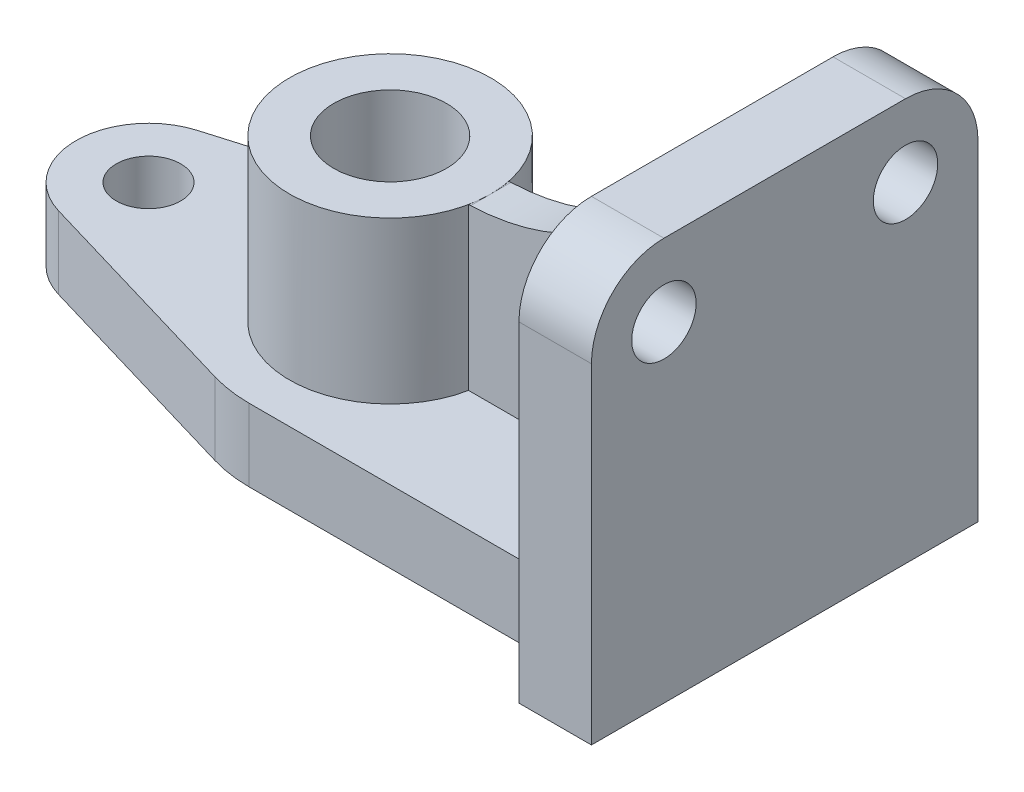
ISO-10303-21;
HEADER;
FILE_DESCRIPTION(('STEP AP214'),'2;1');
FILE_NAME('part.step','',(''),(''),'','','');
FILE_SCHEMA(('AUTOMOTIVE_DESIGN { 1 0 10303 214 1 1 1 1 }'));
ENDSEC;
DATA;
#1=APPLICATION_CONTEXT('core data for automotive mechanical design processes');
#2=APPLICATION_PROTOCOL_DEFINITION('international standard','automotive_design',2000,#1);
#3=PRODUCT_CONTEXT('',#1,'mechanical');
#4=PRODUCT('Part','Part','',(#3));
#5=PRODUCT_RELATED_PRODUCT_CATEGORY('part','',(#4));
#6=PRODUCT_DEFINITION_FORMATION('','',#4);
#7=PRODUCT_DEFINITION_CONTEXT('part definition',#1,'design');
#8=PRODUCT_DEFINITION('design','',#6,#7);
#9=PRODUCT_DEFINITION_SHAPE('','',#8);
#10=(LENGTH_UNIT() NAMED_UNIT(*) SI_UNIT(.MILLI.,.METRE.));
#11=(NAMED_UNIT(*) PLANE_ANGLE_UNIT() SI_UNIT($,.RADIAN.));
#12=(NAMED_UNIT(*) SI_UNIT($,.STERADIAN.) SOLID_ANGLE_UNIT());
#13=UNCERTAINTY_MEASURE_WITH_UNIT(LENGTH_MEASURE(1.E-05),#10,'distance_accuracy_value','');
#14=(GEOMETRIC_REPRESENTATION_CONTEXT(3) GLOBAL_UNCERTAINTY_ASSIGNED_CONTEXT((#13)) GLOBAL_UNIT_ASSIGNED_CONTEXT((#10,
#11,#12)) REPRESENTATION_CONTEXT('',''));
#15=CARTESIAN_POINT('',(0.,0.,0.));
#16=DIRECTION('',(0.,0.,1.));
#17=DIRECTION('',(1.,0.,0.));
#18=AXIS2_PLACEMENT_3D('',#15,#16,#17);
#19=CARTESIAN_POINT('',(0.,82.,30.));
#20=DIRECTION('',(-1.,0.,0.));
#21=DIRECTION('',(0.,0.,1.));
#22=AXIS2_PLACEMENT_3D('',#19,#20,#21);
#23=PLANE('',#22);
#24=CARTESIAN_POINT('',(0.,82.,-30.));
#25=DIRECTION('',(1.,0.,0.));
#26=DIRECTION('',(0.,0.,-1.));
#27=AXIS2_PLACEMENT_3D('',#24,#25,#26);
#28=CIRCLE('',#27,8.);
#29=CARTESIAN_POINT('',(0.,82.,-38.));
#30=VERTEX_POINT('',#29);
#31=EDGE_CURVE('E241',#30,#30,#28,.T.);
#32=ORIENTED_EDGE('',*,*,#31,.T.);
#33=EDGE_LOOP('',(#32));
#34=FACE_BOUND('',#33,.T.);
#35=DIRECTION('',(0.,0.,-1.));
#36=VECTOR('',#35,1.);
#37=CARTESIAN_POINT('',(0.,18.,-35.));
#38=LINE('',#37,#36);
#39=CARTESIAN_POINT('',(0.,18.,-5.));
#40=VERTEX_POINT('',#39);
#41=CARTESIAN_POINT('',(0.,18.,-48.));
#42=VERTEX_POINT('',#41);
#43=EDGE_CURVE('E313',#40,#42,#38,.T.);
#44=ORIENTED_EDGE('',*,*,#43,.F.);
#45=DIRECTION('',(0.,1.,0.));
#46=VECTOR('',#45,1.);
#47=CARTESIAN_POINT('',(0.,82.,-5.));
#48=LINE('',#47,#46);
#49=CARTESIAN_POINT('',(0.,100.,-4.99999999999999));
#50=VERTEX_POINT('',#49);
#51=EDGE_CURVE('E220',#40,#50,#48,.T.);
#52=ORIENTED_EDGE('',*,*,#51,.T.);
#53=DIRECTION('',(0.,0.,1.));
#54=VECTOR('',#53,1.);
#55=CARTESIAN_POINT('',(0.,100.,30.));
#56=LINE('',#55,#54);
#57=CARTESIAN_POINT('',(0.,100.,-30.));
#58=VERTEX_POINT('',#57);
#59=EDGE_CURVE('E278',#58,#50,#56,.T.);
#60=ORIENTED_EDGE('',*,*,#59,.F.);
#61=CARTESIAN_POINT('',(0.,82.,-30.));
#62=DIRECTION('',(1.,0.,0.));
#63=DIRECTION('',(0.,0.,1.));
#64=AXIS2_PLACEMENT_3D('',#61,#62,#63);
#65=CIRCLE('',#64,18.);
#66=CARTESIAN_POINT('',(0.,82.,-48.));
#67=VERTEX_POINT('',#66);
#68=EDGE_CURVE('E280',#67,#58,#65,.T.);
#69=ORIENTED_EDGE('',*,*,#68,.F.);
#70=DIRECTION('',(0.,1.,0.));
#71=VECTOR('',#70,1.);
#72=CARTESIAN_POINT('',(0.,0.,-48.));
#73=LINE('',#72,#71);
#74=EDGE_CURVE('E272',#42,#67,#73,.T.);
#75=ORIENTED_EDGE('',*,*,#74,.F.);
#76=EDGE_LOOP('',(#44,#52,#60,#69,#75));
#77=FACE_BOUND('',#76,.T.);
#78=ADVANCED_FACE('F44',(#34,#77),#23,.T.);
#79=CARTESIAN_POINT('',(-80.,18.,0.));
#80=DIRECTION('',(0.,1.,0.));
#81=DIRECTION('',(0.,0.,1.));
#82=AXIS2_PLACEMENT_3D('',#79,#80,#81);
#83=PLANE('',#82);
#84=CARTESIAN_POINT('',(-140.,18.,0.));
#85=DIRECTION('',(0.,1.,0.));
#86=DIRECTION('',(0.,0.,1.));
#87=AXIS2_PLACEMENT_3D('',#84,#85,#86);
#88=CIRCLE('',#87,8.00000000000001);
#89=CARTESIAN_POINT('',(-140.,18.,8.00000000000001));
#90=VERTEX_POINT('',#89);
#91=EDGE_CURVE('E305',#90,#90,#88,.T.);
#92=ORIENTED_EDGE('',*,*,#91,.F.);
#93=EDGE_LOOP('',(#92));
#94=FACE_BOUND('',#93,.T.);
#95=CARTESIAN_POINT('',(-140.,18.,0.));
#96=DIRECTION('',(0.,1.,0.));
#97=DIRECTION('',(0.,0.,1.));
#98=AXIS2_PLACEMENT_3D('',#95,#96,#97);
#99=CIRCLE('',#98,18.);
#100=CARTESIAN_POINT('',(-145.1,18.,-17.2623868569789));
#101=VERTEX_POINT('',#100);
#102=CARTESIAN_POINT('',(-145.1,18.,17.2623868569789));
#103=VERTEX_POINT('',#102);
#104=EDGE_CURVE('E320',#101,#103,#99,.T.);
#105=ORIENTED_EDGE('',*,*,#104,.T.);
#106=DIRECTION('',(0.959021492054387,0.,0.283333333333333));
#107=VECTOR('',#106,1.);
#108=CARTESIAN_POINT('',(-145.1,18.,17.262386856979));
#109=LINE('',#108,#107);
#110=CARTESIAN_POINT('',(-89.9166666666667,18.,33.5657522219035));
#111=VERTEX_POINT('',#110);
#112=EDGE_CURVE('E317',#103,#111,#109,.T.);
#113=ORIENTED_EDGE('',*,*,#112,.T.);
#114=CARTESIAN_POINT('',(-80.,18.,0.));
#115=DIRECTION('',(0.,1.,0.));
#116=DIRECTION('',(0.,0.,1.));
#117=AXIS2_PLACEMENT_3D('',#114,#115,#116);
#118=CIRCLE('',#117,35.);
#119=CARTESIAN_POINT('',(-80.,18.,35.));
#120=VERTEX_POINT('',#119);
#121=EDGE_CURVE('E321',#111,#120,#118,.T.);
#122=ORIENTED_EDGE('',*,*,#121,.T.);
#123=DIRECTION('',(1.,0.,0.));
#124=VECTOR('',#123,1.);
#125=CARTESIAN_POINT('',(0.,18.,35.));
#126=LINE('',#125,#124);
#127=CARTESIAN_POINT('',(-13.,18.,35.));
#128=VERTEX_POINT('',#127);
#129=EDGE_CURVE('E323',#120,#128,#126,.T.);
#130=ORIENTED_EDGE('',*,*,#129,.T.);
#131=CARTESIAN_POINT('',(-13.,18.,48.));
#132=DIRECTION('',(0.,1.,0.));
#133=DIRECTION('',(0.,0.,1.));
#134=AXIS2_PLACEMENT_3D('',#131,#132,#133);
#135=CIRCLE('',#134,13.);
#136=CARTESIAN_POINT('',(0.,18.,48.));
#137=VERTEX_POINT('',#136);
#138=EDGE_CURVE('E11',#128,#137,#135,.F.);
#139=ORIENTED_EDGE('',*,*,#138,.T.);
#140=CARTESIAN_POINT('',(0.,18.,5.));
#141=VERTEX_POINT('',#140);
#142=EDGE_CURVE('E306',#137,#141,#38,.T.);
#143=ORIENTED_EDGE('',*,*,#142,.T.);
#144=DIRECTION('',(1.,0.,0.));
#145=VECTOR('',#144,1.);
#146=CARTESIAN_POINT('',(-80.,18.,5.));
#147=LINE('',#146,#145);
#148=CARTESIAN_POINT('',(-55.5051025721682,18.,5.));
#149=VERTEX_POINT('',#148);
#150=EDGE_CURVE('E221',#149,#141,#147,.T.);
#151=ORIENTED_EDGE('',*,*,#150,.F.);
#152=CARTESIAN_POINT('',(-80.,18.,0.));
#153=DIRECTION('',(0.,1.,0.));
#154=DIRECTION('',(0.,0.,1.));
#155=AXIS2_PLACEMENT_3D('',#152,#153,#154);
#156=CIRCLE('',#155,25.);
#157=CARTESIAN_POINT('',(-55.5051025721682,18.,-5.));
#158=VERTEX_POINT('',#157);
#159=EDGE_CURVE('E234',#158,#149,#156,.T.);
#160=ORIENTED_EDGE('',*,*,#159,.F.);
#161=DIRECTION('',(1.,0.,0.));
#162=VECTOR('',#161,1.);
#163=CARTESIAN_POINT('',(-80.,18.,-5.));
#164=LINE('',#163,#162);
#165=EDGE_CURVE('E58',#158,#40,#164,.T.);
#166=ORIENTED_EDGE('',*,*,#165,.T.);
#167=ORIENTED_EDGE('',*,*,#43,.T.);
#168=CARTESIAN_POINT('',(-13.,18.,-48.));
#169=DIRECTION('',(0.,1.,0.));
#170=DIRECTION('',(0.,0.,1.));
#171=AXIS2_PLACEMENT_3D('',#168,#169,#170);
#172=CIRCLE('',#171,13.);
#173=CARTESIAN_POINT('',(-13.,18.,-35.));
#174=VERTEX_POINT('',#173);
#175=EDGE_CURVE('E364',#42,#174,#172,.F.);
#176=ORIENTED_EDGE('',*,*,#175,.T.);
#177=DIRECTION('',(-1.,0.,0.));
#178=VECTOR('',#177,1.);
#179=CARTESIAN_POINT('',(0.,18.,-35.));
#180=LINE('',#179,#178);
#181=CARTESIAN_POINT('',(-80.,18.,-35.));
#182=VERTEX_POINT('',#181);
#183=EDGE_CURVE('E309',#174,#182,#180,.T.);
#184=ORIENTED_EDGE('',*,*,#183,.T.);
#185=CARTESIAN_POINT('',(-80.,18.,0.));
#186=DIRECTION('',(0.,1.,0.));
#187=DIRECTION('',(0.,0.,1.));
#188=AXIS2_PLACEMENT_3D('',#185,#186,#187);
#189=CIRCLE('',#188,35.);
#190=CARTESIAN_POINT('',(-89.9166666666667,18.,-33.5657522219035));
#191=VERTEX_POINT('',#190);
#192=EDGE_CURVE('E311',#182,#191,#189,.T.);
#193=ORIENTED_EDGE('',*,*,#192,.T.);
#194=DIRECTION('',(-0.959021492054387,0.,0.283333333333333));
#195=VECTOR('',#194,1.);
#196=CARTESIAN_POINT('',(-145.1,18.,-17.2623868569789));
#197=LINE('',#196,#195);
#198=EDGE_CURVE('E312',#191,#101,#197,.T.);
#199=ORIENTED_EDGE('',*,*,#198,.T.);
#200=EDGE_LOOP('',(#105,#113,#122,#130,#139,#143,#151,#160,#166,#167,#176,#184,#193,#199));
#201=FACE_BOUND('',#200,.T.);
#202=ADVANCED_FACE('F381',(#94,#201),#83,.T.);
#203=CARTESIAN_POINT('',(-80.,0.,0.));
#204=DIRECTION('',(0.,1.,0.));
#205=DIRECTION('',(0.,0.,1.));
#206=AXIS2_PLACEMENT_3D('',#203,#204,#205);
#207=PLANE('',#206);
#208=CARTESIAN_POINT('',(-140.,0.,0.));
#209=DIRECTION('',(0.,1.,0.));
#210=DIRECTION('',(0.,0.,1.));
#211=AXIS2_PLACEMENT_3D('',#208,#209,#210);
#212=CIRCLE('',#211,8.00000000000001);
#213=CARTESIAN_POINT('',(-140.,0.,8.00000000000001));
#214=VERTEX_POINT('',#213);
#215=EDGE_CURVE('E301',#214,#214,#212,.T.);
#216=ORIENTED_EDGE('',*,*,#215,.T.);
#217=EDGE_LOOP('',(#216));
#218=FACE_BOUND('',#217,.T.);
#219=CARTESIAN_POINT('',(-80.,0.,0.));
#220=DIRECTION('',(0.,1.,0.));
#221=DIRECTION('',(0.,0.,1.));
#222=AXIS2_PLACEMENT_3D('',#219,#220,#221);
#223=CIRCLE('',#222,14.);
#224=CARTESIAN_POINT('',(-80.,0.,14.));
#225=VERTEX_POINT('',#224);
#226=EDGE_CURVE('E235',#225,#225,#223,.T.);
#227=ORIENTED_EDGE('',*,*,#226,.T.);
#228=EDGE_LOOP('',(#227));
#229=FACE_BOUND('',#228,.T.);
#230=DIRECTION('',(0.959021492054387,0.,0.283333333333333));
#231=VECTOR('',#230,1.);
#232=CARTESIAN_POINT('',(-145.1,0.,17.262386856979));
#233=LINE('',#232,#231);
#234=CARTESIAN_POINT('',(-145.1,0.,17.2623868569789));
#235=VERTEX_POINT('',#234);
#236=CARTESIAN_POINT('',(-89.9166666666667,0.,33.5657522219035));
#237=VERTEX_POINT('',#236);
#238=EDGE_CURVE('E331',#235,#237,#233,.T.);
#239=ORIENTED_EDGE('',*,*,#238,.F.);
#240=CARTESIAN_POINT('',(-140.,0.,0.));
#241=DIRECTION('',(0.,1.,0.));
#242=DIRECTION('',(0.,0.,1.));
#243=AXIS2_PLACEMENT_3D('',#240,#241,#242);
#244=CIRCLE('',#243,18.);
#245=CARTESIAN_POINT('',(-145.1,0.,-17.2623868569789));
#246=VERTEX_POINT('',#245);
#247=EDGE_CURVE('E335',#246,#235,#244,.T.);
#248=ORIENTED_EDGE('',*,*,#247,.F.);
#249=DIRECTION('',(-0.959021492054387,0.,0.283333333333333));
#250=VECTOR('',#249,1.);
#251=CARTESIAN_POINT('',(-145.1,0.,-17.2623868569789));
#252=LINE('',#251,#250);
#253=CARTESIAN_POINT('',(-89.9166666666667,0.,-33.5657522219035));
#254=VERTEX_POINT('',#253);
#255=EDGE_CURVE('E329',#254,#246,#252,.T.);
#256=ORIENTED_EDGE('',*,*,#255,.F.);
#257=CARTESIAN_POINT('',(-80.,0.,0.));
#258=DIRECTION('',(0.,1.,0.));
#259=DIRECTION('',(0.,0.,1.));
#260=AXIS2_PLACEMENT_3D('',#257,#258,#259);
#261=CIRCLE('',#260,35.);
#262=CARTESIAN_POINT('',(-80.,0.,-35.));
#263=VERTEX_POINT('',#262);
#264=EDGE_CURVE('E327',#263,#254,#261,.T.);
#265=ORIENTED_EDGE('',*,*,#264,.F.);
#266=DIRECTION('',(-1.,0.,0.));
#267=VECTOR('',#266,1.);
#268=CARTESIAN_POINT('',(0.,0.,-35.));
#269=LINE('',#268,#267);
#270=CARTESIAN_POINT('',(-13.,0.,-35.));
#271=VERTEX_POINT('',#270);
#272=EDGE_CURVE('E304',#271,#263,#269,.T.);
#273=ORIENTED_EDGE('',*,*,#272,.F.);
#274=CARTESIAN_POINT('',(-13.,0.,-48.));
#275=DIRECTION('',(0.,1.,0.));
#276=DIRECTION('',(0.,0.,1.));
#277=AXIS2_PLACEMENT_3D('',#274,#275,#276);
#278=CIRCLE('',#277,13.);
#279=CARTESIAN_POINT('',(0.,0.,-48.));
#280=VERTEX_POINT('',#279);
#281=EDGE_CURVE('E361',#271,#280,#278,.T.);
#282=ORIENTED_EDGE('',*,*,#281,.T.);
#283=DIRECTION('',(-1.,0.,0.));
#284=VECTOR('',#283,1.);
#285=CARTESIAN_POINT('',(18.,0.,-48.));
#286=LINE('',#285,#284);
#287=CARTESIAN_POINT('',(18.,0.,-48.));
#288=VERTEX_POINT('',#287);
#289=EDGE_CURVE('E293',#288,#280,#286,.T.);
#290=ORIENTED_EDGE('',*,*,#289,.F.);
#291=DIRECTION('',(0.,0.,-1.));
#292=VECTOR('',#291,1.);
#293=CARTESIAN_POINT('',(18.,0.,48.));
#294=LINE('',#293,#292);
#295=CARTESIAN_POINT('',(18.,0.,48.));
#296=VERTEX_POINT('',#295);
#297=EDGE_CURVE('E256',#296,#288,#294,.T.);
#298=ORIENTED_EDGE('',*,*,#297,.F.);
#299=DIRECTION('',(-1.,0.,0.));
#300=VECTOR('',#299,1.);
#301=CARTESIAN_POINT('',(18.,0.,48.));
#302=LINE('',#301,#300);
#303=CARTESIAN_POINT('',(0.,0.,48.));
#304=VERTEX_POINT('',#303);
#305=EDGE_CURVE('E299',#296,#304,#302,.T.);
#306=ORIENTED_EDGE('',*,*,#305,.T.);
#307=CARTESIAN_POINT('',(-13.,0.,48.));
#308=DIRECTION('',(0.,1.,0.));
#309=DIRECTION('',(0.,0.,1.));
#310=AXIS2_PLACEMENT_3D('',#307,#308,#309);
#311=CIRCLE('',#310,13.);
#312=CARTESIAN_POINT('',(-13.,0.,35.));
#313=VERTEX_POINT('',#312);
#314=EDGE_CURVE('E52',#304,#313,#311,.T.);
#315=ORIENTED_EDGE('',*,*,#314,.T.);
#316=DIRECTION('',(1.,0.,0.));
#317=VECTOR('',#316,1.);
#318=CARTESIAN_POINT('',(0.,0.,35.));
#319=LINE('',#318,#317);
#320=CARTESIAN_POINT('',(-80.,0.,35.));
#321=VERTEX_POINT('',#320);
#322=EDGE_CURVE('E339',#321,#313,#319,.T.);
#323=ORIENTED_EDGE('',*,*,#322,.F.);
#324=CARTESIAN_POINT('',(-80.,0.,0.));
#325=DIRECTION('',(0.,1.,0.));
#326=DIRECTION('',(0.,0.,1.));
#327=AXIS2_PLACEMENT_3D('',#324,#325,#326);
#328=CIRCLE('',#327,35.);
#329=EDGE_CURVE('E336',#237,#321,#328,.T.);
#330=ORIENTED_EDGE('',*,*,#329,.F.);
#331=EDGE_LOOP('',(#239,#248,#256,#265,#273,#282,#290,#298,#306,#315,#323,#330));
#332=FACE_BOUND('',#331,.T.);
#333=ADVANCED_FACE('F369',(#218,#229,#332),#207,.F.);
#334=CARTESIAN_POINT('',(0.,18.,-35.));
#335=DIRECTION('',(0.,0.,1.));
#336=DIRECTION('',(1.,0.,0.));
#337=AXIS2_PLACEMENT_3D('',#334,#335,#336);
#338=PLANE('',#337);
#339=ORIENTED_EDGE('',*,*,#183,.F.);
#340=DIRECTION('',(0.,-1.,0.));
#341=VECTOR('',#340,1.);
#342=CARTESIAN_POINT('',(-13.,18.,-35.));
#343=LINE('',#342,#341);
#344=EDGE_CURVE('E357',#174,#271,#343,.T.);
#345=ORIENTED_EDGE('',*,*,#344,.T.);
#346=ORIENTED_EDGE('',*,*,#272,.T.);
#347=DIRECTION('',(0.,-1.,0.));
#348=VECTOR('',#347,1.);
#349=CARTESIAN_POINT('',(-80.,18.,-35.));
#350=LINE('',#349,#348);
#351=EDGE_CURVE('E355',#182,#263,#350,.T.);
#352=ORIENTED_EDGE('',*,*,#351,.F.);
#353=EDGE_LOOP('',(#339,#345,#346,#352));
#354=FACE_BOUND('',#353,.T.);
#355=ADVANCED_FACE('F459',(#354),#338,.F.);
#356=CARTESIAN_POINT('',(-80.,18.,0.));
#357=DIRECTION('',(0.,-1.,0.));
#358=DIRECTION('',(0.,0.,-1.));
#359=AXIS2_PLACEMENT_3D('',#356,#357,#358);
#360=CYLINDRICAL_SURFACE('',#359,35.);
#361=ORIENTED_EDGE('',*,*,#264,.T.);
#362=DIRECTION('',(0.,-1.,0.));
#363=VECTOR('',#362,1.);
#364=CARTESIAN_POINT('',(-89.9166666666667,18.,-33.5657522219035));
#365=LINE('',#364,#363);
#366=EDGE_CURVE('E352',#191,#254,#365,.T.);
#367=ORIENTED_EDGE('',*,*,#366,.F.);
#368=ORIENTED_EDGE('',*,*,#192,.F.);
#369=ORIENTED_EDGE('',*,*,#351,.T.);
#370=EDGE_LOOP('',(#361,#367,#368,#369));
#371=FACE_BOUND('',#370,.T.);
#372=ADVANCED_FACE('F478',(#371),#360,.T.);
#373=CARTESIAN_POINT('',(-145.1,18.,-17.2623868569789));
#374=DIRECTION('',(0.283333333333333,0.,0.959021492054387));
#375=DIRECTION('',(0.959021492054387,0.,-0.283333333333333));
#376=AXIS2_PLACEMENT_3D('',#373,#374,#375);
#377=PLANE('',#376);
#378=ORIENTED_EDGE('',*,*,#255,.T.);
#379=DIRECTION('',(0.,-1.,0.));
#380=VECTOR('',#379,1.);
#381=CARTESIAN_POINT('',(-145.1,18.,-17.2623868569789));
#382=LINE('',#381,#380);
#383=EDGE_CURVE('E349',#101,#246,#382,.T.);
#384=ORIENTED_EDGE('',*,*,#383,.F.);
#385=ORIENTED_EDGE('',*,*,#198,.F.);
#386=ORIENTED_EDGE('',*,*,#366,.T.);
#387=EDGE_LOOP('',(#378,#384,#385,#386));
#388=FACE_BOUND('',#387,.T.);
#389=ADVANCED_FACE('F472',(#388),#377,.F.);
#390=CARTESIAN_POINT('',(-140.,18.,0.));
#391=DIRECTION('',(0.,-1.,0.));
#392=DIRECTION('',(0.,0.,-1.));
#393=AXIS2_PLACEMENT_3D('',#390,#391,#392);
#394=CYLINDRICAL_SURFACE('',#393,18.);
#395=DIRECTION('',(0.,-1.,0.));
#396=VECTOR('',#395,1.);
#397=CARTESIAN_POINT('',(-145.1,18.,17.2623868569789));
#398=LINE('',#397,#396);
#399=EDGE_CURVE('E347',#103,#235,#398,.T.);
#400=ORIENTED_EDGE('',*,*,#399,.F.);
#401=ORIENTED_EDGE('',*,*,#104,.F.);
#402=ORIENTED_EDGE('',*,*,#383,.T.);
#403=ORIENTED_EDGE('',*,*,#247,.T.);
#404=EDGE_LOOP('',(#400,#401,#402,#403));
#405=FACE_BOUND('',#404,.T.);
#406=ADVANCED_FACE('F467',(#405),#394,.T.);
#407=CARTESIAN_POINT('',(-145.1,18.,17.262386856979));
#408=DIRECTION('',(0.283333333333333,0.,-0.959021492054387));
#409=DIRECTION('',(-0.959021492054387,0.,-0.283333333333333));
#410=AXIS2_PLACEMENT_3D('',#407,#408,#409);
#411=PLANE('',#410);
#412=ORIENTED_EDGE('',*,*,#238,.T.);
#413=DIRECTION('',(0.,-1.,0.));
#414=VECTOR('',#413,1.);
#415=CARTESIAN_POINT('',(-89.9166666666667,18.,33.5657522219035));
#416=LINE('',#415,#414);
#417=EDGE_CURVE('E342',#111,#237,#416,.T.);
#418=ORIENTED_EDGE('',*,*,#417,.F.);
#419=ORIENTED_EDGE('',*,*,#112,.F.);
#420=ORIENTED_EDGE('',*,*,#399,.T.);
#421=EDGE_LOOP('',(#412,#418,#419,#420));
#422=FACE_BOUND('',#421,.T.);
#423=ADVANCED_FACE('F463',(#422),#411,.F.);
#424=CARTESIAN_POINT('',(-80.,18.,0.));
#425=DIRECTION('',(0.,-1.,0.));
#426=DIRECTION('',(0.,0.,-1.));
#427=AXIS2_PLACEMENT_3D('',#424,#425,#426);
#428=CYLINDRICAL_SURFACE('',#427,35.);
#429=ORIENTED_EDGE('',*,*,#329,.T.);
#430=DIRECTION('',(0.,-1.,0.));
#431=VECTOR('',#430,1.);
#432=CARTESIAN_POINT('',(-80.,18.,35.));
#433=LINE('',#432,#431);
#434=EDGE_CURVE('E326',#120,#321,#433,.T.);
#435=ORIENTED_EDGE('',*,*,#434,.F.);
#436=ORIENTED_EDGE('',*,*,#121,.F.);
#437=ORIENTED_EDGE('',*,*,#417,.T.);
#438=EDGE_LOOP('',(#429,#435,#436,#437));
#439=FACE_BOUND('',#438,.T.);
#440=ADVANCED_FACE('F451',(#439),#428,.T.);
#441=CARTESIAN_POINT('',(0.,18.,35.));
#442=DIRECTION('',(0.,0.,-1.));
#443=DIRECTION('',(-1.,0.,0.));
#444=AXIS2_PLACEMENT_3D('',#441,#442,#443);
#445=PLANE('',#444);
#446=ORIENTED_EDGE('',*,*,#322,.T.);
#447=DIRECTION('',(0.,-1.,0.));
#448=VECTOR('',#447,1.);
#449=CARTESIAN_POINT('',(-13.,18.,35.));
#450=LINE('',#449,#448);
#451=EDGE_CURVE('E363',#313,#128,#450,.F.);
#452=ORIENTED_EDGE('',*,*,#451,.T.);
#453=ORIENTED_EDGE('',*,*,#129,.F.);
#454=ORIENTED_EDGE('',*,*,#434,.T.);
#455=EDGE_LOOP('',(#446,#452,#453,#454));
#456=FACE_BOUND('',#455,.T.);
#457=ADVANCED_FACE('F380',(#456),#445,.F.);
#458=CARTESIAN_POINT('',(-140.,18.,0.));
#459=DIRECTION('',(0.,-1.,0.));
#460=DIRECTION('',(0.,0.,-1.));
#461=AXIS2_PLACEMENT_3D('',#458,#459,#460);
#462=CYLINDRICAL_SURFACE('',#461,8.00000000000001);
#463=ORIENTED_EDGE('',*,*,#215,.F.);
#464=EDGE_LOOP('',(#463));
#465=FACE_BOUND('',#464,.T.);
#466=ORIENTED_EDGE('',*,*,#91,.T.);
#467=EDGE_LOOP('',(#466));
#468=FACE_BOUND('',#467,.T.);
#469=ADVANCED_FACE('F437',(#465,#468),#462,.F.);
#470=DIRECTION('',(0.,1.,0.));
#471=VECTOR('',#470,1.);
#472=CARTESIAN_POINT('',(0.,82.,5.));
#473=LINE('',#472,#471);
#474=CARTESIAN_POINT('',(0.,100.,5.00000000000001));
#475=VERTEX_POINT('',#474);
#476=EDGE_CURVE('E67',#141,#475,#473,.T.);
#477=ORIENTED_EDGE('',*,*,#476,.F.);
#478=ORIENTED_EDGE('',*,*,#142,.F.);
#479=DIRECTION('',(0.,-1.,0.));
#480=VECTOR('',#479,1.);
#481=CARTESIAN_POINT('',(0.,0.,48.));
#482=LINE('',#481,#480);
#483=CARTESIAN_POINT('',(0.,82.,48.));
#484=VERTEX_POINT('',#483);
#485=EDGE_CURVE('E269',#484,#137,#482,.T.);
#486=ORIENTED_EDGE('',*,*,#485,.F.);
#487=CARTESIAN_POINT('',(0.,82.,30.));
#488=DIRECTION('',(1.,0.,0.));
#489=DIRECTION('',(0.,0.,1.));
#490=AXIS2_PLACEMENT_3D('',#487,#488,#489);
#491=CIRCLE('',#490,18.);
#492=CARTESIAN_POINT('',(0.,100.,30.));
#493=VERTEX_POINT('',#492);
#494=EDGE_CURVE('E259',#493,#484,#491,.T.);
#495=ORIENTED_EDGE('',*,*,#494,.F.);
#496=EDGE_CURVE('E276',#475,#493,#56,.T.);
#497=ORIENTED_EDGE('',*,*,#496,.F.);
#498=EDGE_LOOP('',(#477,#478,#486,#495,#497));
#499=FACE_BOUND('',#498,.T.);
#500=CARTESIAN_POINT('',(0.,82.,30.));
#501=DIRECTION('',(1.,0.,0.));
#502=DIRECTION('',(0.,0.,-1.));
#503=AXIS2_PLACEMENT_3D('',#500,#501,#502);
#504=CIRCLE('',#503,8.);
#505=CARTESIAN_POINT('',(0.,82.,22.));
#506=VERTEX_POINT('',#505);
#507=EDGE_CURVE('E246',#506,#506,#504,.T.);
#508=ORIENTED_EDGE('',*,*,#507,.T.);
#509=EDGE_LOOP('',(#508));
#510=FACE_BOUND('',#509,.T.);
#511=ADVANCED_FACE('F386',(#499,#510),#23,.T.);
#512=CARTESIAN_POINT('',(18.,82.,30.));
#513=DIRECTION('',(-1.,0.,0.));
#514=DIRECTION('',(0.,0.,1.));
#515=AXIS2_PLACEMENT_3D('',#512,#513,#514);
#516=PLANE('',#515);
#517=ORIENTED_EDGE('',*,*,#297,.T.);
#518=DIRECTION('',(0.,1.,0.));
#519=VECTOR('',#518,1.);
#520=CARTESIAN_POINT('',(18.,0.,-48.));
#521=LINE('',#520,#519);
#522=CARTESIAN_POINT('',(18.,82.,-48.));
#523=VERTEX_POINT('',#522);
#524=EDGE_CURVE('E261',#288,#523,#521,.T.);
#525=ORIENTED_EDGE('',*,*,#524,.T.);
#526=CARTESIAN_POINT('',(18.,82.,-30.));
#527=DIRECTION('',(1.,0.,0.));
#528=DIRECTION('',(0.,0.,1.));
#529=AXIS2_PLACEMENT_3D('',#526,#527,#528);
#530=CIRCLE('',#529,18.);
#531=CARTESIAN_POINT('',(18.,100.,-30.));
#532=VERTEX_POINT('',#531);
#533=EDGE_CURVE('E263',#523,#532,#530,.T.);
#534=ORIENTED_EDGE('',*,*,#533,.T.);
#535=DIRECTION('',(0.,0.,1.));
#536=VECTOR('',#535,1.);
#537=CARTESIAN_POINT('',(18.,100.,30.));
#538=LINE('',#537,#536);
#539=CARTESIAN_POINT('',(18.,100.,30.));
#540=VERTEX_POINT('',#539);
#541=EDGE_CURVE('E264',#532,#540,#538,.T.);
#542=ORIENTED_EDGE('',*,*,#541,.T.);
#543=CARTESIAN_POINT('',(18.,82.,30.));
#544=DIRECTION('',(1.,0.,0.));
#545=DIRECTION('',(0.,0.,1.));
#546=AXIS2_PLACEMENT_3D('',#543,#544,#545);
#547=CIRCLE('',#546,18.);
#548=CARTESIAN_POINT('',(18.,82.,48.));
#549=VERTEX_POINT('',#548);
#550=EDGE_CURVE('E270',#540,#549,#547,.T.);
#551=ORIENTED_EDGE('',*,*,#550,.T.);
#552=DIRECTION('',(0.,-1.,0.));
#553=VECTOR('',#552,1.);
#554=CARTESIAN_POINT('',(18.,0.,48.));
#555=LINE('',#554,#553);
#556=EDGE_CURVE('E254',#549,#296,#555,.T.);
#557=ORIENTED_EDGE('',*,*,#556,.T.);
#558=EDGE_LOOP('',(#517,#525,#534,#542,#551,#557));
#559=FACE_BOUND('',#558,.T.);
#560=CARTESIAN_POINT('',(18.,82.,30.));
#561=DIRECTION('',(1.,0.,0.));
#562=DIRECTION('',(0.,0.,-1.));
#563=AXIS2_PLACEMENT_3D('',#560,#561,#562);
#564=CIRCLE('',#563,8.);
#565=CARTESIAN_POINT('',(18.,82.,22.));
#566=VERTEX_POINT('',#565);
#567=EDGE_CURVE('E248',#566,#566,#564,.T.);
#568=ORIENTED_EDGE('',*,*,#567,.F.);
#569=EDGE_LOOP('',(#568));
#570=FACE_BOUND('',#569,.T.);
#571=CARTESIAN_POINT('',(18.,82.,-30.));
#572=DIRECTION('',(1.,0.,0.));
#573=DIRECTION('',(0.,0.,-1.));
#574=AXIS2_PLACEMENT_3D('',#571,#572,#573);
#575=CIRCLE('',#574,8.);
#576=CARTESIAN_POINT('',(18.,82.,-38.));
#577=VERTEX_POINT('',#576);
#578=EDGE_CURVE('E244',#577,#577,#575,.T.);
#579=ORIENTED_EDGE('',*,*,#578,.F.);
#580=EDGE_LOOP('',(#579));
#581=FACE_BOUND('',#580,.T.);
#582=ADVANCED_FACE('F440',(#559,#570,#581),#516,.F.);
#583=CARTESIAN_POINT('',(18.,0.,48.));
#584=DIRECTION('',(0.,0.,-1.));
#585=DIRECTION('',(-1.,0.,0.));
#586=AXIS2_PLACEMENT_3D('',#583,#584,#585);
#587=PLANE('',#586);
#588=ORIENTED_EDGE('',*,*,#485,.T.);
#589=EDGE_CURVE('E252',#137,#304,#482,.T.);
#590=ORIENTED_EDGE('',*,*,#589,.T.);
#591=ORIENTED_EDGE('',*,*,#305,.F.);
#592=ORIENTED_EDGE('',*,*,#556,.F.);
#593=DIRECTION('',(-1.,0.,0.));
#594=VECTOR('',#593,1.);
#595=CARTESIAN_POINT('',(18.,82.,48.));
#596=LINE('',#595,#594);
#597=EDGE_CURVE('E267',#549,#484,#596,.T.);
#598=ORIENTED_EDGE('',*,*,#597,.T.);
#599=EDGE_LOOP('',(#588,#590,#591,#592,#598));
#600=FACE_BOUND('',#599,.T.);
#601=ADVANCED_FACE('F384',(#600),#587,.F.);
#602=CARTESIAN_POINT('',(18.,0.,-48.));
#603=DIRECTION('',(0.,0.,1.));
#604=DIRECTION('',(1.,0.,0.));
#605=AXIS2_PLACEMENT_3D('',#602,#603,#604);
#606=PLANE('',#605);
#607=EDGE_CURVE('E273',#280,#42,#73,.T.);
#608=ORIENTED_EDGE('',*,*,#607,.T.);
#609=ORIENTED_EDGE('',*,*,#74,.T.);
#610=DIRECTION('',(-1.,0.,0.));
#611=VECTOR('',#610,1.);
#612=CARTESIAN_POINT('',(18.,82.,-48.));
#613=LINE('',#612,#611);
#614=EDGE_CURVE('E295',#523,#67,#613,.T.);
#615=ORIENTED_EDGE('',*,*,#614,.F.);
#616=ORIENTED_EDGE('',*,*,#524,.F.);
#617=ORIENTED_EDGE('',*,*,#289,.T.);
#618=EDGE_LOOP('',(#608,#609,#615,#616,#617));
#619=FACE_BOUND('',#618,.T.);
#620=ADVANCED_FACE('F516',(#619),#606,.F.);
#621=CARTESIAN_POINT('',(18.,82.,-30.));
#622=DIRECTION('',(-1.,0.,0.));
#623=DIRECTION('',(0.,0.,1.));
#624=AXIS2_PLACEMENT_3D('',#621,#622,#623);
#625=CYLINDRICAL_SURFACE('',#624,18.);
#626=ORIENTED_EDGE('',*,*,#68,.T.);
#627=DIRECTION('',(-1.,0.,0.));
#628=VECTOR('',#627,1.);
#629=CARTESIAN_POINT('',(18.,100.,-30.));
#630=LINE('',#629,#628);
#631=EDGE_CURVE('E288',#532,#58,#630,.T.);
#632=ORIENTED_EDGE('',*,*,#631,.F.);
#633=ORIENTED_EDGE('',*,*,#533,.F.);
#634=ORIENTED_EDGE('',*,*,#614,.T.);
#635=EDGE_LOOP('',(#626,#632,#633,#634));
#636=FACE_BOUND('',#635,.T.);
#637=ADVANCED_FACE('F525',(#636),#625,.T.);
#638=CARTESIAN_POINT('',(18.,100.,30.));
#639=DIRECTION('',(0.,-1.,0.));
#640=DIRECTION('',(0.,0.,-1.));
#641=AXIS2_PLACEMENT_3D('',#638,#639,#640);
#642=PLANE('',#641);
#643=DIRECTION('',(-1.,0.,0.));
#644=VECTOR('',#643,1.);
#645=CARTESIAN_POINT('',(18.,100.,30.));
#646=LINE('',#645,#644);
#647=EDGE_CURVE('E286',#540,#493,#646,.T.);
#648=ORIENTED_EDGE('',*,*,#647,.F.);
#649=ORIENTED_EDGE('',*,*,#541,.F.);
#650=ORIENTED_EDGE('',*,*,#631,.T.);
#651=ORIENTED_EDGE('',*,*,#59,.T.);
#652=DIRECTION('',(0.,0.,1.));
#653=VECTOR('',#652,1.);
#654=CARTESIAN_POINT('',(0.,100.,0.));
#655=LINE('',#654,#653);
#656=EDGE_CURVE('E214',#50,#475,#655,.T.);
#657=ORIENTED_EDGE('',*,*,#656,.T.);
#658=ORIENTED_EDGE('',*,*,#496,.T.);
#659=EDGE_LOOP('',(#648,#649,#650,#651,#657,#658));
#660=FACE_BOUND('',#659,.T.);
#661=ADVANCED_FACE('F400',(#660),#642,.F.);
#662=CARTESIAN_POINT('',(18.,82.,30.));
#663=DIRECTION('',(-1.,0.,0.));
#664=DIRECTION('',(0.,0.,1.));
#665=AXIS2_PLACEMENT_3D('',#662,#663,#664);
#666=CYLINDRICAL_SURFACE('',#665,18.);
#667=ORIENTED_EDGE('',*,*,#494,.T.);
#668=ORIENTED_EDGE('',*,*,#597,.F.);
#669=ORIENTED_EDGE('',*,*,#550,.F.);
#670=ORIENTED_EDGE('',*,*,#647,.T.);
#671=EDGE_LOOP('',(#667,#668,#669,#670));
#672=FACE_BOUND('',#671,.T.);
#673=ADVANCED_FACE('F392',(#672),#666,.T.);
#674=CARTESIAN_POINT('',(18.,82.,30.));
#675=DIRECTION('',(-1.,0.,0.));
#676=DIRECTION('',(0.,0.,1.));
#677=AXIS2_PLACEMENT_3D('',#674,#675,#676);
#678=CYLINDRICAL_SURFACE('',#677,8.);
#679=ORIENTED_EDGE('',*,*,#567,.T.);
#680=EDGE_LOOP('',(#679));
#681=FACE_BOUND('',#680,.T.);
#682=ORIENTED_EDGE('',*,*,#507,.F.);
#683=EDGE_LOOP('',(#682));
#684=FACE_BOUND('',#683,.T.);
#685=ADVANCED_FACE('F491',(#681,#684),#678,.F.);
#686=CARTESIAN_POINT('',(18.,82.,-30.));
#687=DIRECTION('',(-1.,0.,0.));
#688=DIRECTION('',(0.,0.,1.));
#689=AXIS2_PLACEMENT_3D('',#686,#687,#688);
#690=CYLINDRICAL_SURFACE('',#689,8.);
#691=ORIENTED_EDGE('',*,*,#578,.T.);
#692=EDGE_LOOP('',(#691));
#693=FACE_BOUND('',#692,.T.);
#694=ORIENTED_EDGE('',*,*,#31,.F.);
#695=EDGE_LOOP('',(#694));
#696=FACE_BOUND('',#695,.T.);
#697=ADVANCED_FACE('F484',(#693,#696),#690,.F.);
#698=CARTESIAN_POINT('',(-13.,18.,-48.));
#699=DIRECTION('',(0.,-1.,0.));
#700=DIRECTION('',(0.,0.,-1.));
#701=AXIS2_PLACEMENT_3D('',#698,#699,#700);
#702=CYLINDRICAL_SURFACE('',#701,13.);
#703=ORIENTED_EDGE('',*,*,#175,.F.);
#704=ORIENTED_EDGE('',*,*,#607,.F.);
#705=ORIENTED_EDGE('',*,*,#281,.F.);
#706=ORIENTED_EDGE('',*,*,#344,.F.);
#707=EDGE_LOOP('',(#703,#704,#705,#706));
#708=FACE_BOUND('',#707,.T.);
#709=ADVANCED_FACE('F483',(#708),#702,.F.);
#710=CARTESIAN_POINT('',(-13.,82.,48.));
#711=DIRECTION('',(0.,-1.,0.));
#712=DIRECTION('',(0.,0.,-1.));
#713=AXIS2_PLACEMENT_3D('',#710,#711,#712);
#714=CYLINDRICAL_SURFACE('',#713,13.);
#715=ORIENTED_EDGE('',*,*,#138,.F.);
#716=ORIENTED_EDGE('',*,*,#451,.F.);
#717=ORIENTED_EDGE('',*,*,#314,.F.);
#718=ORIENTED_EDGE('',*,*,#589,.F.);
#719=EDGE_LOOP('',(#715,#716,#717,#718));
#720=FACE_BOUND('',#719,.T.);
#721=ADVANCED_FACE('F50',(#720),#714,.F.);
#722=CARTESIAN_POINT('',(-80.,58.,0.));
#723=DIRECTION('',(0.,-1.,0.));
#724=DIRECTION('',(0.,0.,-1.));
#725=AXIS2_PLACEMENT_3D('',#722,#723,#724);
#726=CYLINDRICAL_SURFACE('',#725,25.);
#727=ORIENTED_EDGE('',*,*,#159,.T.);
#728=DIRECTION('',(0.,-1.,0.));
#729=VECTOR('',#728,1.);
#730=CARTESIAN_POINT('',(-55.5051025721682,58.,5.));
#731=LINE('',#730,#729);
#732=CARTESIAN_POINT('',(-55.5051025721682,57.9810486761248,5.));
#733=VERTEX_POINT('',#732);
#734=EDGE_CURVE('E226',#149,#733,#731,.F.);
#735=ORIENTED_EDGE('',*,*,#734,.T.);
#736=CARTESIAN_POINT('',(-80.,57.0620061686754,0.));
#737=DIRECTION('',(-0.0374933722263072,0.999296876328101,0.));
#738=DIRECTION('',(-0.999296876328101,-0.0374933722263072,0.));
#739=AXIS2_PLACEMENT_3D('',#736,#737,#738);
#740=ELLIPSE('',#739,25.0175904600664,25.);
#741=CARTESIAN_POINT('',(-55.,58.,0.));
#742=VERTEX_POINT('',#741);
#743=EDGE_CURVE('E203',#733,#742,#740,.T.);
#744=ORIENTED_EDGE('',*,*,#743,.T.);
#745=CARTESIAN_POINT('',(-80.,58.,0.));
#746=DIRECTION('',(0.,1.,0.));
#747=DIRECTION('',(0.,0.,1.));
#748=AXIS2_PLACEMENT_3D('',#745,#746,#747);
#749=CIRCLE('',#748,25.);
#750=EDGE_CURVE('E236',#742,#742,#749,.T.);
#751=ORIENTED_EDGE('',*,*,#750,.F.);
#752=CARTESIAN_POINT('',(-55.5051025721682,57.9810486761248,-5.));
#753=VERTEX_POINT('',#752);
#754=EDGE_CURVE('E228',#742,#753,#740,.T.);
#755=ORIENTED_EDGE('',*,*,#754,.T.);
#756=DIRECTION('',(0.,-1.,0.));
#757=VECTOR('',#756,1.);
#758=CARTESIAN_POINT('',(-55.5051025721682,58.,-5.));
#759=LINE('',#758,#757);
#760=EDGE_CURVE('E219',#158,#753,#759,.F.);
#761=ORIENTED_EDGE('',*,*,#760,.F.);
#762=EDGE_LOOP('',(#727,#735,#744,#751,#755,#761));
#763=FACE_BOUND('',#762,.T.);
#764=ADVANCED_FACE('F409',(#763),#726,.T.);
#765=CARTESIAN_POINT('',(-80.,58.,0.));
#766=DIRECTION('',(0.,1.,0.));
#767=DIRECTION('',(0.,0.,1.));
#768=AXIS2_PLACEMENT_3D('',#765,#766,#767);
#769=PLANE('',#768);
#770=CARTESIAN_POINT('',(-80.,58.,0.));
#771=DIRECTION('',(0.,1.,0.));
#772=DIRECTION('',(0.,0.,1.));
#773=AXIS2_PLACEMENT_3D('',#770,#771,#772);
#774=CIRCLE('',#773,14.);
#775=CARTESIAN_POINT('',(-80.,58.,14.));
#776=VERTEX_POINT('',#775);
#777=EDGE_CURVE('E231',#776,#776,#774,.T.);
#778=ORIENTED_EDGE('',*,*,#777,.F.);
#779=EDGE_LOOP('',(#778));
#780=FACE_BOUND('',#779,.T.);
#781=ORIENTED_EDGE('',*,*,#750,.T.);
#782=EDGE_LOOP('',(#781));
#783=FACE_BOUND('',#782,.T.);
#784=ADVANCED_FACE('F410',(#780,#783),#769,.T.);
#785=CARTESIAN_POINT('',(-80.,0.,0.));
#786=DIRECTION('',(0.,1.,0.));
#787=DIRECTION('',(0.,0.,1.));
#788=AXIS2_PLACEMENT_3D('',#785,#786,#787);
#789=CYLINDRICAL_SURFACE('',#788,14.);
#790=ORIENTED_EDGE('',*,*,#226,.F.);
#791=EDGE_LOOP('',(#790));
#792=FACE_BOUND('',#791,.T.);
#793=ORIENTED_EDGE('',*,*,#777,.T.);
#794=EDGE_LOOP('',(#793));
#795=FACE_BOUND('',#794,.T.);
#796=ADVANCED_FACE('F415',(#792,#795),#789,.F.);
#797=CARTESIAN_POINT('',(-55.,58.,0.));
#798=DIRECTION('',(-0.0374933722263072,0.999296876328101,0.));
#799=DIRECTION('',(-0.999296876328101,-0.0374933722263072,0.));
#800=AXIS2_PLACEMENT_3D('',#797,#798,#799);
#801=PLANE('',#800);
#802=ORIENTED_EDGE('',*,*,#743,.F.);
#803=DIRECTION('',(-0.999296876328101,-0.0374933722263072,0.));
#804=VECTOR('',#803,1.);
#805=CARTESIAN_POINT('',(-55.,58.,5.));
#806=LINE('',#805,#804);
#807=CARTESIAN_POINT('',(-55.,58.,5.));
#808=VERTEX_POINT('',#807);
#809=EDGE_CURVE('E200',#808,#733,#806,.T.);
#810=ORIENTED_EDGE('',*,*,#809,.F.);
#811=DIRECTION('',(0.,0.,1.));
#812=VECTOR('',#811,1.);
#813=CARTESIAN_POINT('',(-55.,58.,0.));
#814=LINE('',#813,#812);
#815=EDGE_CURVE('E187',#742,#808,#814,.T.);
#816=ORIENTED_EDGE('',*,*,#815,.F.);
#817=EDGE_LOOP('',(#802,#810,#816));
#818=FACE_BOUND('',#817,.T.);
#819=ADVANCED_FACE('F199',(#818),#801,.T.);
#820=ORIENTED_EDGE('',*,*,#754,.F.);
#821=CARTESIAN_POINT('',(-55.,58.,-5.));
#822=VERTEX_POINT('',#821);
#823=EDGE_CURVE('E193',#822,#742,#814,.T.);
#824=ORIENTED_EDGE('',*,*,#823,.F.);
#825=DIRECTION('',(-0.999296876328101,-0.0374933722263072,0.));
#826=VECTOR('',#825,1.);
#827=CARTESIAN_POINT('',(-55.,58.,-5.));
#828=LINE('',#827,#826);
#829=EDGE_CURVE('E215',#822,#753,#828,.T.);
#830=ORIENTED_EDGE('',*,*,#829,.T.);
#831=EDGE_LOOP('',(#820,#824,#830));
#832=FACE_BOUND('',#831,.T.);
#833=ADVANCED_FACE('F403',(#832),#801,.T.);
#834=CARTESIAN_POINT('',(-70.,50.,5.));
#835=DIRECTION('',(0.,0.,1.));
#836=DIRECTION('',(1.,0.,0.));
#837=AXIS2_PLACEMENT_3D('',#834,#835,#836);
#838=PLANE('',#837);
#839=ORIENTED_EDGE('',*,*,#734,.F.);
#840=ORIENTED_EDGE('',*,*,#150,.T.);
#841=ORIENTED_EDGE('',*,*,#476,.T.);
#842=CARTESIAN_POINT('',(-57.2496023335784,117.957812579686,5.));
#843=DIRECTION('',(0.,0.,1.));
#844=DIRECTION('',(1.,0.,0.));
#845=AXIS2_PLACEMENT_3D('',#842,#843,#844);
#846=CIRCLE('',#845,60.);
#847=EDGE_CURVE('E195',#808,#475,#846,.T.);
#848=ORIENTED_EDGE('',*,*,#847,.F.);
#849=ORIENTED_EDGE('',*,*,#809,.T.);
#850=EDGE_LOOP('',(#839,#840,#841,#848,#849));
#851=FACE_BOUND('',#850,.T.);
#852=ADVANCED_FACE('F206',(#851),#838,.T.);
#853=CARTESIAN_POINT('',(-70.,50.,-5.));
#854=DIRECTION('',(0.,0.,1.));
#855=DIRECTION('',(1.,0.,0.));
#856=AXIS2_PLACEMENT_3D('',#853,#854,#855);
#857=PLANE('',#856);
#858=ORIENTED_EDGE('',*,*,#165,.F.);
#859=ORIENTED_EDGE('',*,*,#760,.T.);
#860=ORIENTED_EDGE('',*,*,#829,.F.);
#861=CARTESIAN_POINT('',(-57.2496023335784,117.957812579686,-5.));
#862=DIRECTION('',(0.,0.,1.));
#863=DIRECTION('',(1.,0.,0.));
#864=AXIS2_PLACEMENT_3D('',#861,#862,#863);
#865=CIRCLE('',#864,60.);
#866=EDGE_CURVE('E204',#822,#50,#865,.T.);
#867=ORIENTED_EDGE('',*,*,#866,.T.);
#868=ORIENTED_EDGE('',*,*,#51,.F.);
#869=EDGE_LOOP('',(#858,#859,#860,#867,#868));
#870=FACE_BOUND('',#869,.T.);
#871=ADVANCED_FACE('F405',(#870),#857,.F.);
#872=CARTESIAN_POINT('',(-57.2496023335784,117.957812579686,0.));
#873=DIRECTION('',(0.,0.,1.));
#874=DIRECTION('',(1.,0.,0.));
#875=AXIS2_PLACEMENT_3D('',#872,#873,#874);
#876=CYLINDRICAL_SURFACE('',#875,60.);
#877=ORIENTED_EDGE('',*,*,#656,.F.);
#878=ORIENTED_EDGE('',*,*,#866,.F.);
#879=ORIENTED_EDGE('',*,*,#823,.T.);
#880=ORIENTED_EDGE('',*,*,#815,.T.);
#881=ORIENTED_EDGE('',*,*,#847,.T.);
#882=EDGE_LOOP('',(#877,#878,#879,#880,#881));
#883=FACE_BOUND('',#882,.T.);
#884=ADVANCED_FACE('F190',(#883),#876,.F.);
#885=CLOSED_SHELL('',(#78,#202,#333,#355,#372,#389,#406,#423,#440,#457,#469,#511,#582,#601,#620,
#637,#661,#673,#685,#697,#709,#721,#764,#784,#796,#819,#833,#852,#871,#884));
#886=MANIFOLD_SOLID_BREP('B2',#885);
#887=ADVANCED_BREP_SHAPE_REPRESENTATION('',(#18,#886),#14);
#888=SHAPE_DEFINITION_REPRESENTATION(#9,#887);
ENDSEC;
END-ISO-10303-21;
